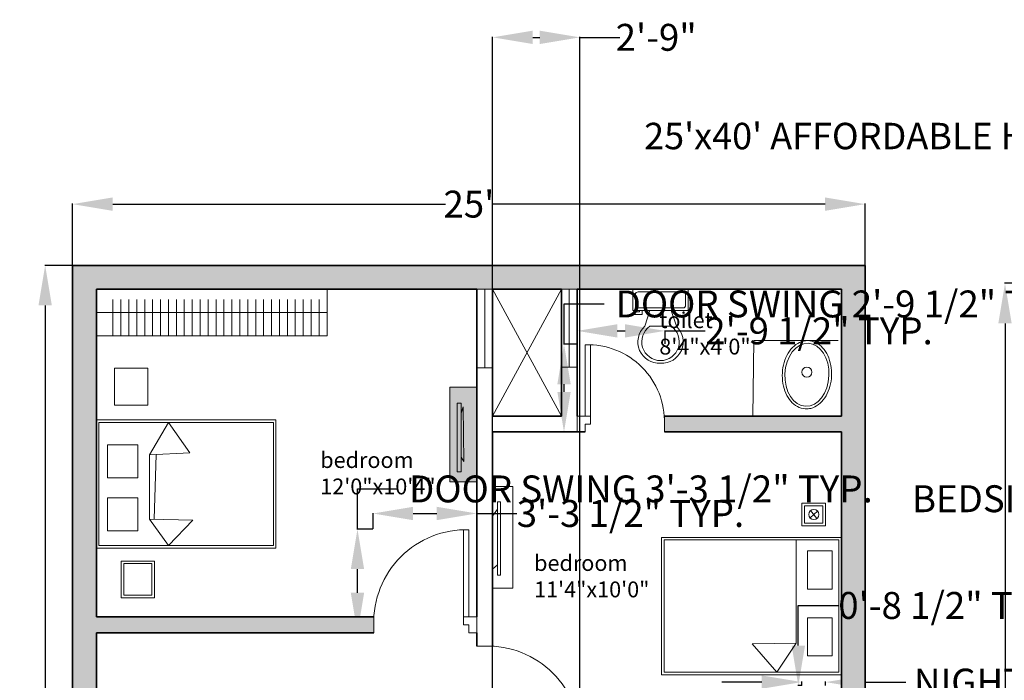
# Model space of a CAD drawing. Units: inches. Extents: x 19 to 15718, y 7 to 930.
# Tile 5 of 11: x 14871 to 15243, y 680 to 930. Entities that reach past the tile are written whole.
import ezdxf

# ---------------------------------------------------------------- set-up
doc = ezdxf.new("R2010")
doc.units = ezdxf.units.IN
doc.header["$MEASUREMENT"] = 0
for name, color, linetype, lineweight in [('A-ANNO-DIMS', 2, 'Continuous', 18), ('A-ANNO-TEXT', 7, 'Continuous', 25), ('A-AREA-IDEN', 7, 'Continuous', 18), ('A-DOOR', 4, 'Continuous', 20), ('A-FLOR-CASE', 8, 'Continuous', 18), ('A-FLOR-FIXT', 9, 'Continuous', 18), ('A-FLOR-OPEN', 8, 'Continuous', 13), ('A-FURN', 8, 'Continuous', 18), ('A-GLAZ', 4, 'Continuous', 18), ('A-WALL', 7, 'Continuous', 35)]:
    doc.layers.add(name, color=color, linetype=linetype, lineweight=lineweight)
doc.layers.add('A-FURN-PATT', color=18, linetype='Continuous', lineweight=13, true_color=0x000000)
doc.layers.add('A-WALL-PATT', color=18, linetype='Continuous', lineweight=13, true_color=0x000000)
doc.styles.add('Annotative', font='arial.ttf')
doc.styles.get("Standard").update_dxf_attribs({"font": 'arial.ttf'})
doc.dimstyles.get("Standard").update_dxf_attribs({"dimtxt": 10.18, "dimasz": 15.18, "dimexe": 0.18, "dimexo": 0.0625, "dimgap": 0.09, "dimtad": 0, "dimtih": 1, "dimtoh": 1, "dimdec": 0, "dimzin": 0, "dimdsep": 46, "dimlunit": 3, "dimtxsty": 'Standard', "dimcen": 0.09, "dimadec": 0, "dimazin": 0, "dimtfac": 1, "dimtdec": 0, "dimtofl": 0, "dimtmove": 0, "dimatfit": 3, "dimfxl": 1, "dimtolj": 1, "dimtzin": 0, "dimarcsym": 0})

# ---------------------------------------------------------------- blocks, each defined once
blk = doc.blocks.new('*U2')
for p, q in [((9.5, -6), (9.5, -2)), ((-10, -8.5), (-8, -8.5)), ((-10, -9.5), (-10, -8.5)), ((-7, -9.5), (-10, -9.5)), ((-8, -8.5), (-8, -8)), ((-7, -8), (-7, -9.5)), ((-4, -8), (-6, -14)), ((4, -8), (6, -14)), ((4, -14), (-4, -14))]:
    blk.add_line(p, q)
blk.add_lwpolyline([(10.5, -8), (10.5, 0), (-10.5, 0), (-10.5, -8)], close=True)
for points in [[(-9.5, -2), (-9.5, -6)], [(8.5, -1), (-8.5, -1)], [(-8.5, -7), (8.5, -7)]]:
    blk.add_lwpolyline(points)
for centre, radius, start, end in [((-8.625, -1.875), 0.8839, 81.8699, 188.1301), ((8.625, -1.875), 0.8839, 351.8699, 98.1301), ((-8.625, -6.125), 0.8839, 171.869898, 278.1301), ((8.625, -6.125), 0.8839, 261.8699, 8.1301), ((-0.4772, -19.9188), 8.0953, 133.01722, 273.38), ((0.0374, -19.8731), 7.127, 124.50543, 269.7), ((-0.0373, -19.8731), 7.127, 270.3, 55.4946), ((0.4773, -19.9188), 8.0953, 266.62, 46.9828)]:
    blk.add_arc(centre, radius, start, end)
blk = doc.blocks.new('*D5')
at = {"layer": 'A-ANNO-DIMS', "color": 0, "lineweight": -2, "transparency": 16777216}
for p, q in [((14890.84, 837.06), (14890.84, 860.41)), ((14906.02, 860.23), (15032.02, 860.23)), ((15175.66, 860.23), (15049.65, 860.23)), ((15190.84, 837.06), (15190.84, 860.41))]:
    blk.add_line(p, q, dxfattribs=at)
at = {"layer": 'A-ANNO-DIMS', "color": 0, "transparency": 16777216}
for points in [[(14906.02, 862.76), (14906.02, 857.7), (14890.84, 860.23)], [(15175.66, 862.76), (15175.66, 857.7), (15190.84, 860.23)]]:
    blk.add_solid(points, dxfattribs=at)
at = {"layer": 'Defpoints', "color": 0, "transparency": 16777216}
for p in [(15190.84, 860.23), (14890.84, 837), (15190.84, 837)]:
    blk.add_point(p, dxfattribs=at)
at = {"layer": 'A-ANNO-DIMS', "color": 0, "transparency": 16777216, "insert": (15040.84, 860.23), "char_height": 10.18, "attachment_point": 5}
blk.add_mtext("\\A1;25'", dxfattribs=at)
blk = doc.blocks.new('*D6')
at = {"layer": 'A-ANNO-DIMS', "color": 0, "lineweight": -2, "transparency": 16777216}
for p, q in [((14890.77, 837.06), (14880.28, 837.06)), ((14880.46, 821.88), (14880.46, 602.31)), ((14880.46, 372.18), (14880.46, 591.74)), ((14890.77, 357), (14880.28, 357))]:
    blk.add_line(p, q, dxfattribs=at)
at = {"layer": 'A-ANNO-DIMS', "color": 0, "transparency": 16777216}
for points in [[(14877.93, 821.88), (14882.99, 821.88), (14880.46, 837.06)], [(14877.93, 372.18), (14882.99, 372.18), (14880.46, 357)]]:
    blk.add_solid(points, dxfattribs=at)
at = {"layer": 'Defpoints', "color": 0, "transparency": 16777216}
for p in [(14890.84, 837.06), (14880.46, 357), (14890.84, 357)]:
    blk.add_point(p, dxfattribs=at)
at = {"layer": 'A-ANNO-DIMS', "color": 0, "transparency": 16777216, "insert": (14880.46, 597.03), "char_height": 10.18, "attachment_point": 5}
blk.add_mtext("\\A1;40'", dxfattribs=at)
blk = doc.blocks.new('*D17')
at = {"layer": 'A-ANNO-DIMS', "color": 0, "lineweight": -2, "transparency": 16777216}
for p, q in [((15266.62, 830.27), (15243.58, 830.27)), ((15243.76, 815.09), (15243.76, 595.52)), ((15243.76, 365.38), (15243.76, 584.95)), ((15266.62, 350.2), (15243.58, 350.2))]:
    blk.add_line(p, q, dxfattribs=at)
at = {"layer": 'A-ANNO-DIMS', "color": 0, "transparency": 16777216}
for points in [[(15241.23, 815.09), (15246.29, 815.09), (15243.76, 830.27)], [(15241.23, 365.38), (15246.29, 365.38), (15243.76, 350.2)]]:
    blk.add_solid(points, dxfattribs=at)
at = {"layer": 'Defpoints', "color": 0, "transparency": 16777216}
for p in [(15266.68, 830.27), (15243.76, 350.2), (15266.68, 350.2)]:
    blk.add_point(p, dxfattribs=at)
at = {"layer": 'A-ANNO-DIMS', "color": 0, "transparency": 16777216, "insert": (15243.76, 590.24), "char_height": 10.18, "attachment_point": 5}
blk.add_mtext("\\A1;40'", dxfattribs=at)
blk = doc.blocks.new('DOOR-SWING-36IN')
for p, q in [((34.01, 3), (34.01, 39)), ((36.01, 6), (36.01, 39)), ((0.01, 6), (0.01, 0)), ((34.01, 6), (39.01, 6)), ((39.01, 6), (39.01, 0)), ((34.01, 3), (36.01, 3)), ((36.01, 3), (36.01, 0))]:
    blk.add_line(p, q)
blk.add_arc((35.01, 4), 35.01, 88.3634, 181.6366)
blk = doc.blocks.new('DOOR-SWING-30IN')
for p, q in [((3, 6), (3, 33)), ((5, 3), (5, 33)), ((0, 6), (0, 0)), ((0, 6), (5, 6)), ((33, 6), (33, 0)), ((3, 3), (3, 0)), ((5, 3), (3, 3))]:
    blk.add_line(p, q)
blk.add_arc((4, 4), 29.02, 358.0251, 91.9749)
blk = doc.blocks.new('NIGHTSTAND-SQUARE')
for p, q in [((5.89, 5.61), (3.09, 2.97)), ((3.32, 5.82), (5.66, 2.76)), ((3.09, 2.97), (3.09, 2.97))]:
    blk.add_line(p, q)
for points in [[(0, 8.58), (8.98, 8.58), (8.98, 0), (0, 0)], [(1, 7.58), (7.98, 7.58), (7.98, 1), (1, 1)]]:
    blk.add_lwpolyline(points, close=True)
blk.add_circle((4.49, 4.29), 1.92)
blk = doc.blocks.new('*D34')
at = {"layer": 'A-ANNO-DIMS', "color": 0, "lineweight": -2, "transparency": 16777216}
for p, q in [((14998.67, 737.27), (14998.67, 752.45)), ((14998.67, 752.45), (15013.85, 752.45)), ((15004.5, 737.27), (14998.49, 737.27)), ((14998.67, 713.18), (14998.67, 722.09)), ((15004.5, 698), (14998.49, 698))]:
    blk.add_line(p, q, dxfattribs=at)
at = {"layer": 'A-ANNO-DIMS', "color": 0, "transparency": 16777216}
for points in [[(14996.14, 722.09), (15001.2, 722.09), (14998.67, 737.27)], [(14996.14, 713.18), (15001.2, 713.18), (14998.67, 698)]]:
    blk.add_solid(points, dxfattribs=at)
at = {"layer": 'Defpoints', "color": 0, "transparency": 16777216}
for p in [(14998.67, 737.27), (15004.56, 737.27), (15004.56, 698)]:
    blk.add_point(p, dxfattribs=at)
at = {"layer": 'A-ANNO-DIMS', "color": 0, "transparency": 16777216, "insert": (15105.95, 752.45), "char_height": 10.18, "attachment_point": 5}
blk.add_mtext('\\A1;DOOR SWING 3\'-3 1/2" TYP.', dxfattribs=at)
blk = doc.blocks.new('*D35')
at = {"layer": 'A-ANNO-DIMS', "color": 0, "lineweight": -2, "transparency": 16777216}
for p, q in [((15004.56, 737.33), (15004.56, 743.34)), ((15019.74, 743.16), (15028.66, 743.16)), ((15043.84, 737.33), (15043.84, 743.34)), ((15043.84, 743.16), (15059.02, 743.16))]:
    blk.add_line(p, q, dxfattribs=at)
at = {"layer": 'A-ANNO-DIMS', "color": 0, "transparency": 16777216}
for points in [[(15019.74, 745.69), (15019.74, 740.63), (15004.56, 743.16)], [(15028.66, 745.69), (15028.66, 740.63), (15043.84, 743.16)]]:
    blk.add_solid(points, dxfattribs=at)
at = {"layer": 'Defpoints', "color": 0, "transparency": 16777216}
for p in [(15043.84, 743.16), (15004.56, 737.27), (15043.84, 737.27)]:
    blk.add_point(p, dxfattribs=at)
at = {"layer": 'A-ANNO-DIMS', "color": 0, "transparency": 16777216, "insert": (15101.99, 743.16), "char_height": 10.18, "attachment_point": 5}
blk.add_mtext('\\A1;3\'-3 1/2" TYP.', dxfattribs=at)
blk = doc.blocks.new('*D38')
at = {"layer": 'A-ANNO-DIMS', "color": 0, "lineweight": -2, "transparency": 16777216}
for p, q in [((15293.05, 769.31), (15293.05, 784.49)), ((15291.5, 754.13), (15293.23, 754.13)), ((15291.5, 743.35), (15293.23, 743.35)), ((15293.05, 728.17), (15293.05, 712.99))]:
    blk.add_line(p, q, dxfattribs=at)
at = {"layer": 'A-ANNO-DIMS', "color": 0, "transparency": 16777216}
for points in [[(15290.52, 769.31), (15295.58, 769.31), (15293.05, 754.13)], [(15290.52, 728.17), (15295.58, 728.17), (15293.05, 743.35)]]:
    blk.add_solid(points, dxfattribs=at)
at = {"layer": 'Defpoints', "color": 0, "transparency": 16777216}
for p in [(15291.44, 754.13), (15293.05, 754.13), (15291.44, 743.35)]:
    blk.add_point(p, dxfattribs=at)
at = {"layer": 'A-ANNO-DIMS', "color": 0, "transparency": 16777216, "insert": (15293.05, 748.74), "char_height": 10.18, "attachment_point": 5}
blk.add_mtext('\\A1;BEDSIDE LAMP 0\'-11" TYP.', dxfattribs=at)
blk = doc.blocks.new('*D48')
at = {"layer": 'A-ANNO-DIMS', "color": 0, "lineweight": -2, "transparency": 16777216}
for p, q in [((15076.85, 807.27), (15076.85, 822.45)), ((15076.85, 822.45), (15092.03, 822.45)), ((15081.77, 807.27), (15076.67, 807.27)), ((15076.85, 789.18), (15076.85, 792.09)), ((15081.77, 774), (15076.67, 774))]:
    blk.add_line(p, q, dxfattribs=at)
at = {"layer": 'A-ANNO-DIMS', "color": 0, "transparency": 16777216}
for points in [[(15074.32, 792.09), (15079.38, 792.09), (15076.85, 807.27)], [(15074.32, 789.18), (15079.38, 789.18), (15076.85, 774)]]:
    blk.add_solid(points, dxfattribs=at)
at = {"layer": 'Defpoints', "color": 0, "transparency": 16777216}
for p in [(15076.85, 807.27), (15081.84, 807.27), (15081.84, 774)]:
    blk.add_point(p, dxfattribs=at)
at = {"layer": 'A-ANNO-DIMS', "color": 0, "transparency": 16777216, "insert": (15184.13, 822.45), "char_height": 10.18, "attachment_point": 5}
blk.add_mtext('\\A1;DOOR SWING 2\'-9 1/2" TYP.', dxfattribs=at)
blk = doc.blocks.new('*D49')
at = {"layer": 'A-ANNO-DIMS', "color": 0, "lineweight": -2, "transparency": 16777216}
for p, q in [((15081.84, 807.34), (15081.84, 812.44)), ((15115.11, 807.34), (15115.11, 812.44)), ((15097.02, 812.26), (15099.93, 812.26)), ((15115.11, 812.26), (15130.29, 812.26))]:
    blk.add_line(p, q, dxfattribs=at)
at = {"layer": 'A-ANNO-DIMS', "color": 0, "transparency": 16777216}
for points in [[(15097.02, 814.79), (15097.02, 809.73), (15081.84, 812.26)], [(15099.93, 814.79), (15099.93, 809.73), (15115.11, 812.26)]]:
    blk.add_solid(points, dxfattribs=at)
at = {"layer": 'Defpoints', "color": 0, "transparency": 16777216}
for p in [(15115.11, 812.26), (15081.84, 807.27), (15115.11, 807.27)]:
    blk.add_point(p, dxfattribs=at)
at = {"layer": 'A-ANNO-DIMS', "color": 0, "transparency": 16777216, "insert": (15173.36, 812.26), "char_height": 10.18, "attachment_point": 5}
blk.add_mtext('\\A1;2\'-9 1/2" TYP.', dxfattribs=at)
blk = doc.blocks.new('*D56')
at = {"layer": 'A-ANNO-DIMS', "color": 0, "lineweight": -2, "transparency": 16777216}
for p, q in [((15151.7, 679.35), (15136.52, 679.35)), ((15166.88, 678.06), (15166.88, 679.53)), ((15175.86, 678.06), (15175.86, 679.53)), ((15191.04, 679.35), (15206.22, 679.35))]:
    blk.add_line(p, q, dxfattribs=at)
at = {"layer": 'A-ANNO-DIMS', "color": 0, "transparency": 16777216}
for points in [[(15151.7, 681.88), (15151.7, 676.82), (15166.88, 679.35)], [(15191.04, 681.88), (15191.04, 676.82), (15175.86, 679.35)]]:
    blk.add_solid(points, dxfattribs=at)
at = {"layer": 'Defpoints', "color": 0, "transparency": 16777216}
for p in [(15175.86, 679.35), (15166.88, 678), (15175.86, 678)]:
    blk.add_point(p, dxfattribs=at)
at = {"layer": 'A-ANNO-DIMS', "color": 0, "transparency": 16777216, "insert": (15285.29, 679.35), "char_height": 10.18, "attachment_point": 5}
blk.add_mtext('\\A1;NIGHTSTAND 0\'-9" TYP.', dxfattribs=at)
blk = doc.blocks.new('*D57')
at = {"layer": 'A-ANNO-DIMS', "color": 0, "lineweight": -2, "transparency": 16777216}
for p, q in [((15165.53, 693.18), (15165.53, 708.36)), ((15165.53, 708.36), (15180.71, 708.36)), ((15166.82, 678), (15165.35, 678)), ((15166.82, 669.42), (15165.35, 669.42)), ((15165.53, 654.24), (15165.53, 639.06))]:
    blk.add_line(p, q, dxfattribs=at)
at = {"layer": 'A-ANNO-DIMS', "color": 0, "transparency": 16777216}
for points in [[(15163, 693.18), (15168.06, 693.18), (15165.53, 678)], [(15163, 654.24), (15168.06, 654.24), (15165.53, 669.42)]]:
    blk.add_solid(points, dxfattribs=at)
at = {"layer": 'Defpoints', "color": 0, "transparency": 16777216}
for p in [(15165.53, 678), (15166.88, 678), (15166.88, 669.42)]:
    blk.add_point(p, dxfattribs=at)
at = {"layer": 'A-ANNO-DIMS', "color": 0, "transparency": 16777216, "insert": (15223.69, 708.36), "char_height": 10.18, "attachment_point": 5}
blk.add_mtext('\\A1;0\'-8 1/2" TYP.', dxfattribs=at)
blk = doc.blocks.new('*D58')
at = {"layer": 'A-ANNO-DIMS', "color": 0, "lineweight": -2, "transparency": 16777216}
for p, q in [((15278.41, 688.79), (15278.41, 703.97)), ((15280.87, 673.61), (15278.23, 673.61)), ((15280.87, 656.82), (15278.23, 656.82)), ((15278.41, 641.64), (15278.41, 626.46))]:
    blk.add_line(p, q, dxfattribs=at)
at = {"layer": 'A-ANNO-DIMS', "color": 0, "transparency": 16777216}
for points in [[(15275.88, 688.79), (15280.94, 688.79), (15278.41, 673.61)], [(15275.88, 641.64), (15280.94, 641.64), (15278.41, 656.82)]]:
    blk.add_solid(points, dxfattribs=at)
at = {"layer": 'Defpoints', "color": 0, "transparency": 16777216}
for p in [(15278.41, 673.61), (15280.93, 673.61), (15280.93, 656.82)]:
    blk.add_point(p, dxfattribs=at)
at = {"layer": 'A-ANNO-DIMS', "color": 0, "transparency": 16777216, "insert": (15278.41, 665.21), "char_height": 10.18, "attachment_point": 5}
blk.add_mtext('\\A1;NIGHTSTAND 1\'-5" TYP.', dxfattribs=at)
blk = doc.blocks.new('*D78')
at = {"layer": 'A-ANNO-DIMS', "color": 0, "lineweight": -2, "transparency": 16777216}
for p, q in [((15049.84, 534.06), (15049.84, 923.53)), ((15065.02, 923.35), (15067.65, 923.35)), ((15082.83, 534.06), (15082.83, 923.53)), ((15082.83, 923.35), (15098.01, 923.35))]:
    blk.add_line(p, q, dxfattribs=at)
at = {"layer": 'A-ANNO-DIMS', "color": 0, "transparency": 16777216}
for points in [[(15065.02, 925.88), (15065.02, 920.82), (15049.84, 923.35)], [(15067.65, 925.88), (15067.65, 920.82), (15082.83, 923.35)]]:
    blk.add_solid(points, dxfattribs=at)
at = {"layer": 'Defpoints', "color": 0, "transparency": 16777216}
for p in [(15082.83, 923.35), (15049.84, 534), (15082.83, 534)]:
    blk.add_point(p, dxfattribs=at)
at = {"layer": 'A-ANNO-DIMS', "color": 0, "transparency": 16777216, "insert": (15111.72, 923.35), "char_height": 10.18, "attachment_point": 5}
blk.add_mtext('\\A1;2\'-9"', dxfattribs=at)

msp = doc.modelspace()

# ---------------------------------------------------------------- hatches: boundary and pattern name
at = {"layer": 'A-FURN-PATT'}
h = msp.add_hatch(color=256, dxfattribs=at)
h.dxf.hatch_style = 1
h.paths.add_polyline_path([(15033.67, 755.14), (15043.84, 755.14), (15043.84, 790.9), (15033.67, 790.9)])
at = {"layer": 'A-WALL-PATT'}
h = msp.add_hatch(color=256, dxfattribs=at)
h.dxf.hatch_style = 1
h.paths.add_polyline_path([(15190.84, 837), (14890.84, 837), (14890.84, 357), (14899.84, 357), (14899.84, 366), (14899.84, 528), (14904.84, 528), (14904.84, 534), (14899.84, 534), (14899.84, 698), (15004.84, 698), (15004.84, 701, -0.014283), (15004.84, 703), (15004.84, 704), (14899.84, 704), (14899.84, 828), (14987.26, 828), (15043.84, 828), (15049.84, 828), (15075.84, 828), (15081.84, 828), (15181.84, 828), (15181.84, 780), (15114.84, 780), (15114.84, 779, -0.017236), (15114.84, 777), (15114.84, 774), (15181.84, 774), (15181.84, 654), (15181.84, 648), (15181.84, 596), (15190.84, 596)])
h.paths.add_polyline_path([(15190.84, 590), (15181.84, 590), (15181.84, 470), (15181.84, 464), (15181.84, 361.43), (14991.9, 361.43), (14991.5, 357), (15190.84, 357)], flags=0)
h.paths.add_polyline_path([(15152.29, 608), (15146.29, 608), (15146.29, 596), (15049.84, 596), (15049.84, 590), (15152.29, 590)], flags=17)
h.paths.add_polyline_path([(15049.84, 615), (15048.84, 615, -0.017236), (15046.84, 615), (15043.84, 615), (15043.84, 596), (15049.84, 596)], flags=17)
edge = h.paths.add_edge_path(flags=17)
edge.add_line((15152.29, 654), (15049.84, 654))
edge.add_line((15049.84, 654), (15043.84, 654))
edge.add_line((15043.84, 654), (15043.84, 648))
edge.add_line((15043.84, 648), (15049.84, 648))
edge.add_line((15049.84, 648), (15075.84, 648))
edge.add_line((15075.84, 648), (15081.84, 648))
edge.add_line((15081.84, 648), (15117.26, 648))
edge.add_spline(control_points=[(15117.26, 648), (15117.59, 648.02), (15117.94, 648.03), (15118.71, 648.04), (15119.15, 648.02), (15119.59, 648)], knot_values=[1.499122, 1.499122, 1.499122, 1.499122, 1.618335, 1.618335, 1.770388, 1.770388, 1.770388, 1.770388], degree=3, periodic=0)
edge.add_spline(control_points=[(15127.99, 642.93), (15128, 643.28), (15127.95, 643.62), (15127.73, 644.26), (15127.57, 644.57), (15127.16, 645.13), (15126.92, 645.39), (15126.04, 646.16), (15125.28, 646.6), (15123.53, 647.31), (15122.55, 647.59), (15120.88, 647.88), (15120.24, 647.95), (15119.59, 648)], knot_values=[0, 0, 0, 0, 0.172075, 0.172075, 0.344149, 0.344149, 0.516224, 0.516224, 0.894541, 0.894541, 1.272858, 1.272858, 1.499122, 1.499122, 1.499122, 1.499122], degree=3, periodic=0)
edge.add_line((15119.59, 648), (15146.29, 648))
edge.add_line((15146.29, 648), (15146.29, 636))
edge.add_line((15146.29, 636), (15152.29, 636))
edge.add_line((15152.29, 636), (15152.29, 654))
h.paths.add_polyline_path([(15132.35, 430.4), (15123.35, 430.4), (15123.35, 396.8), (15027.77, 396.8), (15027.77, 387.8), (15132.35, 387.8)], flags=17)
h.paths.add_polyline_path([(15132.35, 464), (15123.35, 464), (15123.35, 430.4), (15132.35, 430.4)], flags=17)
h.paths.add_polyline_path([(15275.68, 583.59), (15276.07, 583.2), (15276.65, 583.2), (15280.6, 587.16), (15278.55, 589.2), (15275.68, 589.2), (15275.68, 601.2), (15266.68, 601.2), (15266.68, 350.2), (15275.68, 350.2), (15275.68, 359.2), (15275.68, 457.2), (15413.68, 457.2), (15413.68, 471.04), (15407.68, 471.04), (15407.68, 463.2), (15275.68, 463.2)])

# ---------------------------------------------------------------- linework, layer by layer
at = {"layer": 'A-DOOR'}
msp.add_line((15040.84, 698), (15043.84, 698), dxfattribs=at)
at = {"layer": 'A-FLOR-CASE'}
for p, q in [((14906.14, 824.19), (14906.14, 810.35)), ((14909.14, 824.19), (14909.14, 810.35)), ((14912.14, 824.19), (14912.14, 810.35)), ((14915.14, 824.19), (14915.14, 810.35)), ((14918.14, 824.19), (14918.14, 810.35)), ((14921.14, 824.19), (14921.14, 810.35)), ((14924.14, 824.19), (14924.14, 810.35)), ((14927.14, 824.19), (14927.14, 810.35)), ((14930.14, 824.19), (14930.14, 810.35)), ((14933.14, 824.19), (14933.14, 810.35)), ((14936.14, 824.19), (14936.14, 810.35)), ((14939.14, 824.19), (14939.14, 810.35)), ((14942.14, 824.19), (14942.14, 810.35)), ((14945.14, 824.19), (14945.14, 810.35)), ((14948.14, 824.19), (14948.14, 810.35)), ((14951.14, 824.19), (14951.14, 810.35)), ((14954.14, 824.19), (14954.14, 810.35)), ((14957.14, 824.19), (14957.14, 810.35)), ((14960.14, 824.19), (14960.14, 810.35)), ((14960.14, 824.19), (14960.14, 810.35)), ((14960.14, 824.19), (14960.14, 810.35)), ((14963.14, 824.19), (14963.14, 810.35)), ((14966.14, 824.19), (14966.14, 810.35)), ((14969.14, 824.19), (14969.14, 810.35)), ((14972.14, 824.19), (14972.14, 810.35)), ((14975.14, 824.19), (14975.14, 810.35)), ((14978.14, 824.19), (14978.14, 810.35)), ((14981.14, 824.19), (14981.14, 810.35)), ((14984.14, 824.19), (14984.14, 810.35)), ((14899.84, 819.17), (14987.26, 819.17))]:
    msp.add_line(p, q, dxfattribs=at)
msp.add_lwpolyline([(14899.84, 828), (14987.26, 828), (14987.26, 810.35), (14899.84, 810.35)], close=True, dxfattribs=at)
at = {"layer": 'A-FLOR-FIXT'}
for p, q in [((15181.84, 810.63), (15181.84, 810.63)), ((15148.69, 808.58), (15148.31, 780)), ((15148.69, 808.58), (15180.65, 808.58))]:
    msp.add_line(p, q, dxfattribs=at)
msp.add_circle((15168.79, 796.65), 1.91, dxfattribs=at)
msp.add_ellipse((15168.79, 795.65), major_axis=(-0.48, -11.93), ratio=0.698055, dxfattribs=at)
msp.add_open_spline([(15168.28, 782.72), (15168.94, 782.7), (15169.6, 782.77), (15171.27, 783.19), (15172.25, 783.68), (15174.04, 785.04), (15174.84, 785.91), (15176.21, 787.92), (15176.77, 789.07), (15177.62, 791.54), (15177.91, 792.85), (15178.18, 795.54), (15178.16, 796.9), (15177.83, 799.55), (15177.51, 800.83), (15176.6, 803.2), (15176, 804.28), (15174.57, 806.13), (15173.74, 806.91), (15171.89, 808.04), (15170.89, 808.41), (15168.82, 808.66), (15167.76, 808.54), (15165.75, 807.85), (15164.8, 807.28), (15163.09, 805.79), (15162.33, 804.86), (15161.05, 802.75), (15160.54, 801.56), (15159.79, 799.04), (15159.56, 797.71), (15159.41, 795.02), (15159.48, 793.67), (15159.92, 791.06), (15160.29, 789.8), (15161.3, 787.52), (15161.94, 786.49), (15163.42, 784.77), (15164.26, 784.08), (15166.09, 783.1), (15167.08, 782.8), (15168.15, 782.73), (15168.21, 782.73), (15168.28, 782.72)], degree=3, knots=[0, 0, 0, 0, 0.202926, 0.202926, 0.523413, 0.523413, 0.8439, 0.8439, 1.164388, 1.164388, 1.484875, 1.484875, 1.805363, 1.805363, 2.12585, 2.12585, 2.446337, 2.446337, 2.766184, 2.766184, 3.086031, 3.086031, 3.405878, 3.405878, 3.725725, 3.725725, 4.045572, 4.045572, 4.365419, 4.365419, 4.685266, 4.685266, 5.005113, 5.005113, 5.32496, 5.32496, 5.644807, 5.644807, 5.954508, 5.954508, 6.264208, 6.264208, 6.283185, 6.283185, 6.283185, 6.283185], dxfattribs=at)
at = {"layer": 'A-FLOR-OPEN'}
for p, q in [((15049.84, 828), (15075.84, 780)), ((15075.84, 828), (15049.84, 780))]:
    msp.add_line(p, q, dxfattribs=at)
at = {"layer": 'A-FURN'}
for p, q in [((15037.92, 781.07), (15038.7, 783.51)), ((15038.7, 783.51), (15038.94, 762.84)), ((14920.01, 765.36), (14927.19, 777.64)), ((14927.19, 777.64), (14935.26, 766.1)), ((14935.26, 766.1), (14920.01, 765.36)), ((14920.01, 741.06), (14920.01, 765.36)), ((14922.48, 765.48), (14921.75, 741.01)), ((15038.94, 762.84), (15037.92, 764.51)), ((15051.64, 744.82), (15049.84, 742.2)), ((15049.84, 742.2), (15049.84, 722.11)), ((14920.01, 741.06), (14927.12, 731.01)), ((14936.36, 740.58), (14920.01, 741.06)), ((14927.12, 731.01), (14936.36, 740.58)), ((15164.71, 733.13), (15164.71, 694.1)), ((15049.84, 722.11), (15051.64, 723.74)), ((15148.08, 693.82), (15164.71, 694.1)), ((15157.39, 683.05), (15148.08, 693.82)), ((15164.71, 694.1), (15157.39, 683.05)), ((15164.71, 694.1), (15164.71, 694.1))]:
    msp.add_line(p, q, dxfattribs=at)
for points in [[(14906.77, 798.1), (14919.29, 798.1), (14919.29, 784.21), (14906.77, 784.21)], [(15043.84, 790.9), (15033.67, 790.9), (15033.67, 755.14), (15043.84, 755.14)], [(15037.92, 784.87), (15036.35, 784.87), (15036.35, 758.94), (15037.92, 758.94)], [(14899.84, 778.64), (14967.83, 778.64), (14967.83, 730.01), (14899.84, 730.01)], [(14900.84, 777.64), (14966.83, 777.64), (14966.83, 731.01), (14900.84, 731.01)], [(14915.55, 769.16), (14904.05, 769.16), (14904.05, 756.66), (14915.55, 756.66)], [(15049.84, 753.31), (15057.45, 753.31), (15057.45, 714.92), (15049.84, 714.92)], [(14915.55, 749.13), (14904.05, 749.13), (14904.05, 736.63), (14915.55, 736.63)], [(15051.64, 747.59), (15052.78, 747.59), (15052.78, 719.82), (15051.64, 719.82)], [(15181.84, 734.13), (15113.76, 734.13), (15113.76, 682.05), (15181.84, 682.05)], [(15180.84, 733.13), (15114.76, 733.13), (15114.76, 683.05), (15180.84, 683.05)], [(15168.99, 729.03), (15178.29, 729.03), (15178.29, 714.55), (15168.99, 714.55)], [(14909.29, 725.17), (14921.81, 725.17), (14921.81, 711.28), (14909.29, 711.28)], [(14910.29, 724.17), (14920.81, 724.17), (14920.81, 712.28), (14910.29, 712.28)], [(15168.99, 703.73), (15178.29, 703.73), (15178.29, 689.25), (15168.99, 689.25)]]:
    msp.add_lwpolyline(points, close=True, dxfattribs=at)
at = {"layer": 'A-GLAZ'}
for p, q in [((15043.84, 828), (15049.84, 828)), ((15046.84, 828), (15046.84, 798.24)), ((15075.84, 828), (15081.84, 828)), ((15078.84, 828), (15078.84, 798.47)), ((15043.84, 798.24), (15049.84, 798.24)), ((15075.84, 798.47), (15081.84, 798.47))]:
    msp.add_line(p, q, dxfattribs=at)
at = {"layer": 'A-WALL'}
for p, q in [((14890.84, 357), (14890.84, 837)), ((14890.84, 837), (15190.84, 837)), ((15190.84, 837), (15190.84, 357)), ((14899.84, 828), (15043.84, 828)), ((14899.84, 704), (14899.84, 828)), ((15043.84, 704), (15043.84, 828)), ((15049.84, 780), (15049.84, 828)), ((15049.84, 828), (15075.84, 828)), ((15075.84, 828), (15075.84, 780)), ((15075.84, 828), (15075.84, 780)), ((15081.84, 828), (15081.84, 780)), ((15081.84, 828), (15081.84, 780)), ((15081.84, 828), (15181.84, 828)), ((15181.84, 828), (15181.84, 780)), ((15049.84, 780), (15075.84, 780)), ((15114.78, 780), (15181.84, 780)), ((15049.84, 774), (15084.84, 774)), ((15049.84, 692.95), (15049.84, 774)), ((15114.84, 774), (15181.84, 774)), ((15181.84, 774), (15181.84, 654)), ((14899.84, 704), (15004.88, 704)), ((14899.84, 698), (15004.84, 698)), ((14899.84, 534), (14899.84, 698)), ((15043.84, 693), (15043.84, 698))]:
    msp.add_line(p, q, dxfattribs=at)

# ---------------------------------------------------------------- block references
at = {"layer": 'A-DOOR'}
for name, p in [('DOOR-SWING-30IN', (15081.84, 774)), ('DOOR-SWING-36IN', (15004.83, 698))]:
    msp.add_blockref(name, p, dxfattribs=at)
at = {"layer": 'A-DOOR', "rotation": 269.9999999999929}
msp.add_blockref('DOOR-SWING-36IN', (15043.84, 693), dxfattribs=at)
at = {"layer": 'A-FLOR-FIXT'}
msp.add_blockref('*U2', (15113.38, 828), dxfattribs=at)
at = {"layer": 'A-FURN'}
msp.add_blockref('NIGHTSTAND-SQUARE', (15166.88, 738.48), dxfattribs=at)

# ---------------------------------------------------------------- texts
at = {"layer": 'A-ANNO-TEXT', "insert": (15107.17, 891), "char_height": 10, "attachment_point": 1}
msp.add_mtext_dynamic_manual_height_columns("25'x40' AFFORDABLE HOUSE DESIGN", width=556.6952, gutter_width=1, heights=[0], dxfattribs=at)
at = {"layer": 'A-AREA-IDEN', "char_height": 6, "width": 68.1983, "attachment_point": 1, "style": 'Annotative'}
for s, insert in [('toilet\\P8\'4"x4\'0"', (15112.91, 819.32)), ('bedroom\\P12\'0"x10\'4"', (14984.58, 766.38)), ('bedroom\\P11\'4"x10\'0"', (15065.53, 727.42))]:
    msp.add_mtext(s, dxfattribs=dict(at, insert=insert))

# ---------------------------------------------------------------- dimensions: what is measured, and where the dimension line sits
at = {"layer": 'A-ANNO-DIMS'}
for base, p1, p2, override, picture, middle in [((15082.83, 923.35), (15049.84, 534), (15082.83, 534), {"dimdec": 1, "dimlfac": 1, "dimrnd": 0, "dimzin": 1, "dimdsep": 46, "dimlunit": 4, "dimfrac": 2}, '*D78', (15111.72, 923.35)), ((15190.84, 860.23), (14890.84, 837), (15190.84, 837), {"dimclrd": 0, "dimclre": 0, "dimclrt": 0}, '*D5', (15040.84, 860.23))]:
    dim = msp.add_linear_dim(base=base, p1=p1, p2=p2, dimstyle='Standard', override=override, dxfattribs=at)
    dim.commit()
    dim.dimension.update_dxf_attribs({"geometry": picture, "text_midpoint": middle})
for base, p1, p2, text, picture, middle in [((15076.85, 807.27), (15081.84, 774), (15081.84, 807.27), 'DOOR SWING <> TYP.', '*D48', (15184.13, 822.45)), ((14998.67, 737.27), (15004.56, 698), (15004.56, 737.27), 'DOOR SWING <> TYP.', '*D34', (15105.95, 752.45)), ((15293.05, 754.13), (15291.44, 743.35), (15291.44, 754.13), 'BEDSIDE LAMP <> TYP.', '*D38', (15293.05, 748.74)), ((15165.53, 678), (15166.88, 669.42), (15166.88, 678), '<> TYP.', '*D57', (15223.69, 708.36)), ((15278.41, 673.61), (15280.93, 656.82), (15280.93, 673.61), 'NIGHTSTAND <> TYP.', '*D58', (15278.41, 665.21))]:
    dim = msp.add_linear_dim(base=base, p1=p1, p2=p2, angle=90, text=text, dimstyle='Standard', override={"dimdec": 1, "dimlfac": 1, "dimrnd": 0, "dimzin": 1, "dimdsep": 46, "dimlunit": 4, "dimfrac": 2}, dxfattribs=at)
    dim.commit()
    dim.dimension.update_dxf_attribs({"geometry": picture, "text_midpoint": middle})
for base, p1, p2, picture, middle in [((14880.46, 357), (14890.84, 837.06), (14890.84, 357), '*D6', (14880.46, 597.03)), ((15243.76, 350.2), (15266.68, 830.27), (15266.68, 350.2), '*D17', (15243.76, 590.24))]:
    dim = msp.add_linear_dim(base=base, p1=p1, p2=p2, angle=90, dimstyle='Standard', override={"dimclrd": 0, "dimclre": 0, "dimclrt": 0}, dxfattribs=at)
    dim.commit()
    dim.dimension.update_dxf_attribs({"geometry": picture, "text_midpoint": middle})
for base, p1, p2, text, picture, middle in [((15115.11, 812.26), (15081.84, 807.27), (15115.11, 807.27), '<> TYP.', '*D49', (15173.36, 812.26)), ((15043.84, 743.16), (15004.56, 737.27), (15043.84, 737.27), '<> TYP.', '*D35', (15101.99, 743.16)), ((15175.86, 679.35), (15166.88, 678), (15175.86, 678), 'NIGHTSTAND <> TYP.', '*D56', (15285.29, 679.35))]:
    dim = msp.add_linear_dim(base=base, p1=p1, p2=p2, text=text, dimstyle='Standard', override={"dimdec": 1, "dimlfac": 1, "dimrnd": 0, "dimzin": 1, "dimdsep": 46, "dimlunit": 4, "dimfrac": 2}, dxfattribs=at)
    dim.commit()
    dim.dimension.update_dxf_attribs({"geometry": picture, "text_midpoint": middle})

doc.saveas('drawing.dxf')
